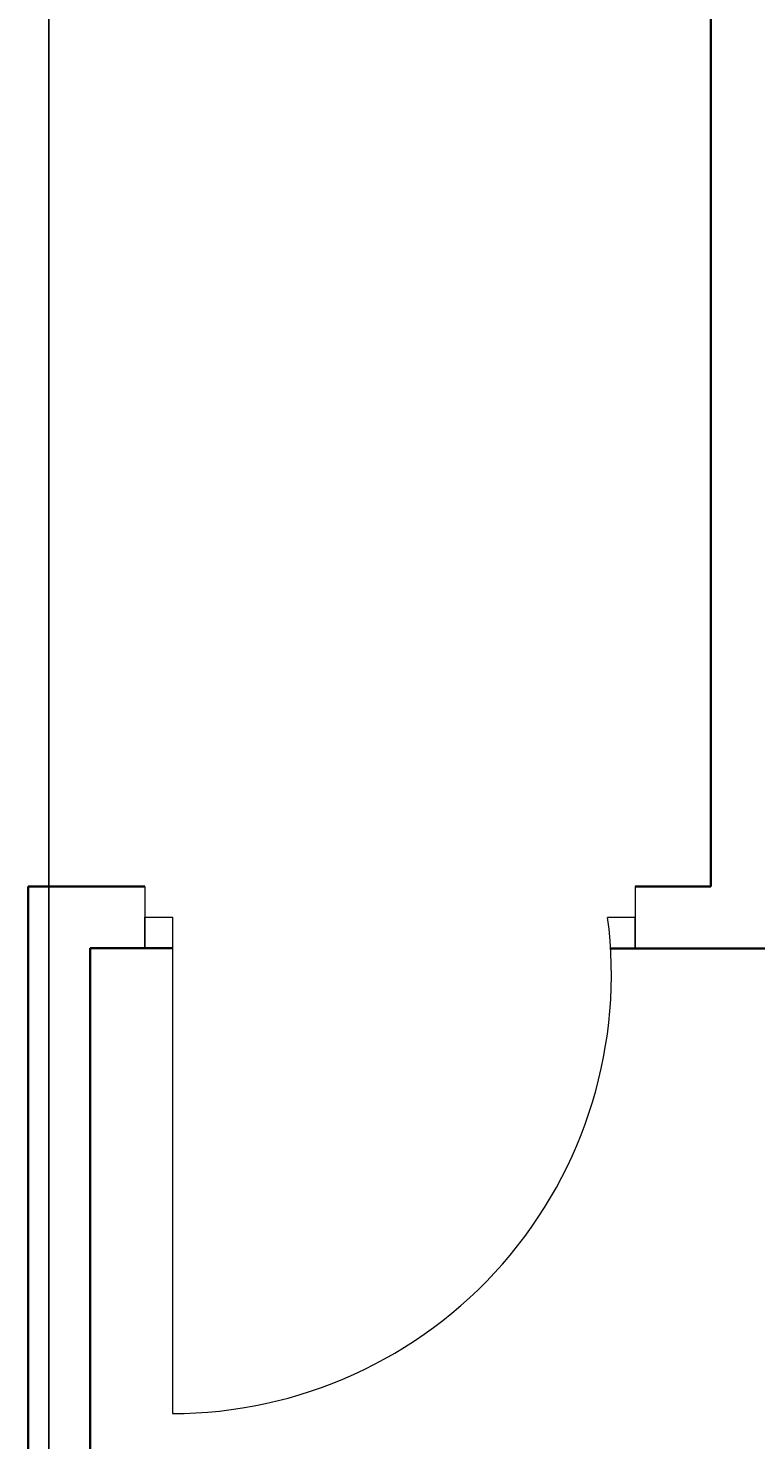
# Model space of a CAD drawing. Units: inches. Extents: x 1088 to 1703, y 668 to 1875.
# Tile 27 of 45: x 1436 to 1489, y 1504 to 1606. Entities that reach past the tile are written whole.
import ezdxf

# ---------------------------------------------------------------- set-up
doc = ezdxf.new("R2010")
doc.units = ezdxf.units.IN
for name, color, linetype, lineweight in [('A-ANNO-DIMS', 2, 'Continuous', 18), ('A-DOOR', 4, 'Continuous', 18), ('A-WALL', 7, 'Continuous', 35)]:
    doc.layers.add(name, color=color, linetype=linetype, lineweight=lineweight)
doc.styles.get("Standard").update_dxf_attribs({"font": 'arial.ttf'})
doc.dimstyles.get("Standard").update_dxf_attribs({"dimtxt": 0.18, "dimasz": 0.18, "dimexe": 0.18, "dimexo": 0.0625, "dimgap": 0.09, "dimtad": 0, "dimtih": 1, "dimtoh": 1, "dimdec": 4, "dimzin": 0, "dimdsep": 46, "dimtxsty": 'Standard', "dimcen": 0.09, "dimadec": 0, "dimazin": 0, "dimtfac": 1, "dimtdec": 4, "dimtofl": 0, "dimtmove": 0, "dimatfit": 3, "dimfxl": 1, "dimtolj": 1, "dimtzin": 0, "dimarcsym": 0})

# ---------------------------------------------------------------- blocks, each defined once
blk = doc.blocks.new('*D38')
at = {"layer": 'A-ANNO-DIMS', "color": 0, "lineweight": -2, "transparency": 16777216}
for p, q in [((1317.34, 1736.94), (1317.34, 725.55)), ((1437.34, 1736.94), (1437.34, 725.55)), ((1317.52, 725.73), (1377.06, 725.73)), ((1437.16, 725.73), (1377.62, 725.73))]:
    blk.add_line(p, q, dxfattribs=at)
at = {"layer": 'A-ANNO-DIMS', "color": 0, "transparency": 16777216}
for points in [[(1317.52, 725.76), (1317.52, 725.7), (1317.34, 725.73)], [(1437.16, 725.76), (1437.16, 725.7), (1437.34, 725.73)]]:
    blk.add_solid(points, dxfattribs=at)
at = {"layer": 'Defpoints', "color": 0, "transparency": 16777216}
for p in [(1317.34, 1737.01), (1437.34, 1737.01), (1437.34, 725.73)]:
    blk.add_point(p, dxfattribs=at)
at = {"layer": 'A-ANNO-DIMS', "color": 0, "transparency": 16777216, "insert": (1377.34, 725.73), "char_height": 0.18, "attachment_point": 5}
blk.add_mtext('\\A1;120', dxfattribs=at)

msp = doc.modelspace()

# ---------------------------------------------------------------- linework, layer by layer
at = {"layer": 'A-DOOR'}
for p, q in [((1444.295, 1544.058), (1444.293, 1539.581)), ((1479.858, 1544.058), (1479.855, 1539.561)), ((1444.293, 1539.581), (1444.294, 1541.82)), ((1444.294, 1541.82), (1446.294, 1541.82)), ((1446.294, 1541.82), (1446.294, 1505.82)), ((1479.856, 1541.81), (1477.856, 1541.81)), ((1479.855, 1539.561), (1479.856, 1541.81))]:
    msp.add_line(p, q, dxfattribs=at)
msp.add_arc((1446.294, 1537.654), 31.835, 270, 7.50023, dxfattribs=at)
at = {"layer": 'A-WALL'}
for p, q in [((1485.345, 1608.558), (1485.345, 1604.058)), ((1485.345, 1604.058), (1485.345, 1544.058)), ((1435.845, 1544.058), (1435.845, 1538.5)), ((1444.295, 1544.058), (1435.845, 1544.058)), ((1485.345, 1544.058), (1479.858, 1544.058)), ((1435.845, 1419.558), (1435.845, 1539.558)), ((1440.345, 1419.558), (1440.345, 1539.583)), ((1446.294, 1539.58), (1440.345, 1539.583)), ((1485.345, 1539.558), (1478.071, 1539.562)), ((1485.345, 1539.558), (1560.928, 1539.558))]:
    msp.add_line(p, q, dxfattribs=at)

# ---------------------------------------------------------------- dimensions: what is measured, and where the dimension line sits
at = {"layer": 'A-ANNO-DIMS'}
dim = msp.add_linear_dim(base=(1437.345, 725.729), p1=(1317.345, 1737.007), p2=(1437.345, 1737.007), dimstyle='Standard', override={"dimdec": 0, "dimlfac": 1, "dimrnd": 0, "dimzin": 0, "dimdsep": 46, "dimlunit": 2}, dxfattribs=at)
dim.commit()
dim.dimension.update_dxf_attribs({"geometry": '*D38', "text_midpoint": (1377.345, 725.729)})

doc.saveas('drawing.dxf')
